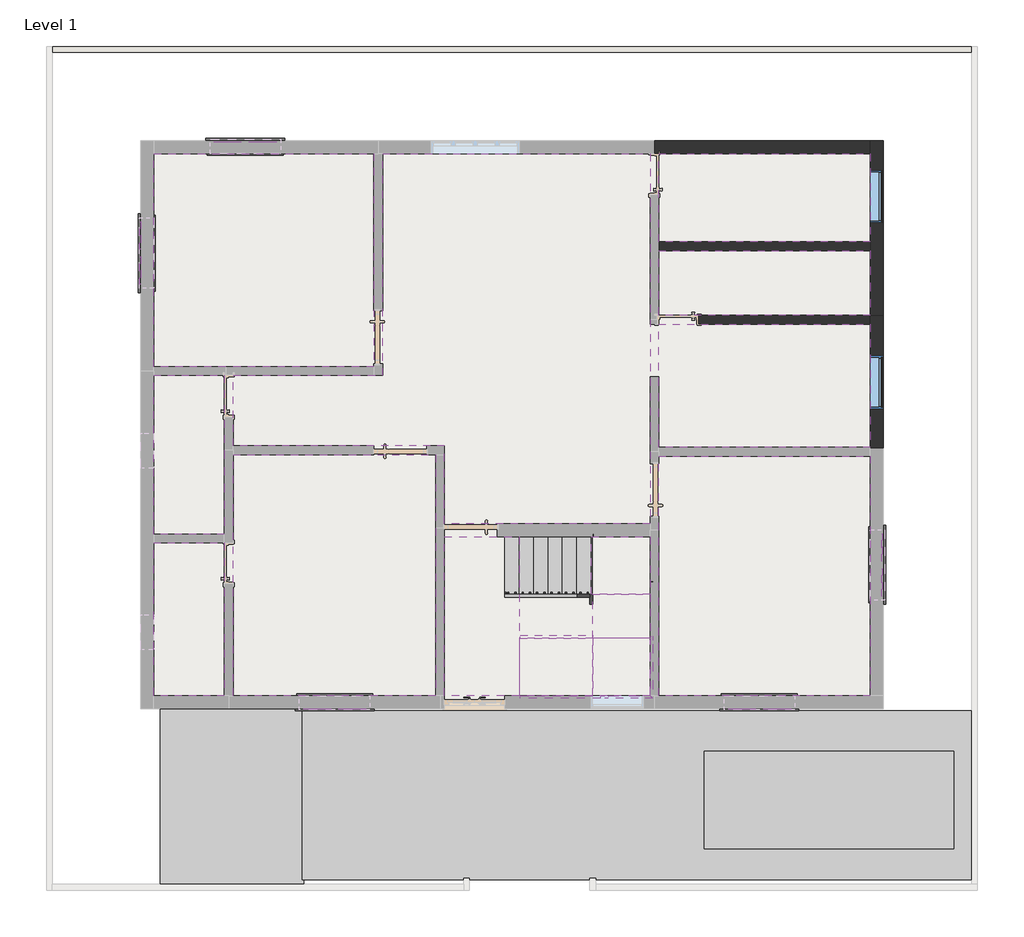
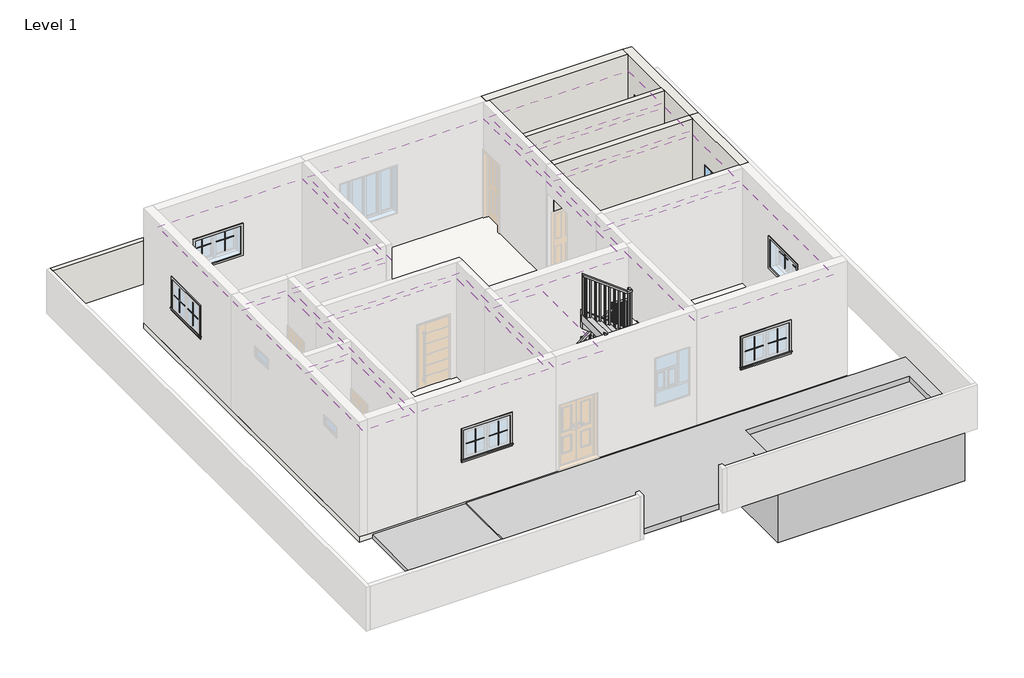
# One storey, part 2 of 2: 22 proxies, 10 coverings, 10 members, 6 walls, 3 slabs, 3 stair flights, 2 windows, 1 railing.
"""IFC4 building model written with IfcOpenShell, lengths in millimetres."""

from ifc_helpers import new_model, si_unit, frame, origin, origin_with_axes, place, context, project, spatial, polyline, outline, extrude, faceted_brep, transform, mapped, element, save
from components import generic_models_1_generic_models_1_4ef364dd, m_muntin_pattern_2x2_m_muntin_pattern_2x2_8d9e5da3, m_muntin_pattern_2x2_m_muntin_pattern_2x2_32a0f80e, m_trim_window_exterior_flat_with_sill_3a557199, m_trim_window_exterior_flat_with_sill_1a4b2e7c, m_trim_window_interior_flat_picture_frame_580345df, m_trim_window_interior_flat_picture_frame_7ff13b15, swimming_pool_swimming_pool_f5703ba1, non_monolithic_landing_f8b46ba6, non_monolithic_landing_0691aa35, stair_flight_50mm_tread_13mm_riser_519f3169, stair_flight_50mm_tread_13mm_riser_ecc54b48, stair_flight_50mm_tread_13mm_riser_ab1ff6a1, m_window_casement_double_sash_variable_3_661e274a

model = new_model("IFC4")

# Units and contexts
model_context = context("Model", 3, world=origin())
ifc_project = project(units=[si_unit("LENGTHUNIT", "METRE", prefix="MILLI")], contexts=[model_context])

# Site, building, storey
site = spatial("IfcSite", under=ifc_project)
building = spatial("IfcBuilding", under=site)
storey = spatial("IfcBuildingStorey", under=building, Name="Level 1", Elevation=0.0)

# Proxies
placement = place(None, origin())
generic_models_1_generic_models_1_shape = generic_models_1_generic_models_1_4ef364dd(model_context)
element("IfcBuildingElementProxy", 1, Name="Generic Models 1 : Generic Models 1", ObjectType="Generic Models 1 : Generic Models 1", at=placement, inside=storey, context=model_context, shape_type="MappedRepresentation", body=[
    mapped(generic_models_1_generic_models_1_shape, transform((0.0, 0.0, 0.0), x_axis=(1.0, 0.0, 0.0), y_axis=(0.0, 1.0, 0.0), z_axis=(0.0, 0.0, 1.0))),
])
m_muntin_pattern_2x2_m_muntin_pattern_2x2_shape = m_muntin_pattern_2x2_m_muntin_pattern_2x2_8d9e5da3(model_context)
element("IfcBuildingElementProxy", 2, Name="M_Muntin Pattern_2x2 : M_Muntin Pattern_2x2", ObjectType="M_Muntin Pattern_2x2 : M_Muntin Pattern_2x2", at=placement, inside=storey, context=model_context, shape_type="MappedRepresentation", body=[
    mapped(m_muntin_pattern_2x2_m_muntin_pattern_2x2_shape, transform((-16781.6669909, 5340.5131491, 1289.05), x_axis=(1.0, 0.0, 0.0), y_axis=(0.0, 1.0, 0.0), z_axis=(0.0, 0.0, 1.0))),
])
element("IfcBuildingElementProxy", 3, Name="M_Muntin Pattern_2x2 : M_Muntin Pattern_2x2", ObjectType="M_Muntin Pattern_2x2 : M_Muntin Pattern_2x2", at=placement, inside=storey, context=model_context, shape_type="MappedRepresentation", body=[
    mapped(m_muntin_pattern_2x2_m_muntin_pattern_2x2_shape, transform((-18281.8544909, 3098.9631491, 1289.05), x_axis=(0.0, 1.0, 0.0), y_axis=(-1.0, 0.0, 0.0), z_axis=(0.0, 0.0, 1.0))),
])
element("IfcBuildingElementProxy", 4, Name="M_Muntin Pattern_2x2 : M_Muntin Pattern_2x2", ObjectType="M_Muntin Pattern_2x2 : M_Muntin Pattern_2x2", at=placement, inside=storey, context=model_context, shape_type="MappedRepresentation", body=[
    mapped(m_muntin_pattern_2x2_m_muntin_pattern_2x2_shape, transform((-5448.5044909, -1687.3493509, 1289.05), x_axis=(0.0, -1.0, 0.0), y_axis=(1.0, 0.0, 0.0), z_axis=(0.0, 0.0, 1.0))),
])
element("IfcBuildingElementProxy", 5, Name="M_Muntin Pattern_2x2 : M_Muntin Pattern_2x2", ObjectType="M_Muntin Pattern_2x2 : M_Muntin Pattern_2x2", at=placement, inside=storey, context=model_context, shape_type="MappedRepresentation", body=[
    mapped(m_muntin_pattern_2x2_m_muntin_pattern_2x2_shape, transform((-7283.6544909, -4470.2368509, 1289.05), x_axis=(-1.0, 0.0, 0.0), y_axis=(0.0, -1.0, 0.0), z_axis=(0.0, 0.0, 1.0))),
])
element("IfcBuildingElementProxy", 6, Name="M_Muntin Pattern_2x2 : M_Muntin Pattern_2x2", ObjectType="M_Muntin Pattern_2x2 : M_Muntin Pattern_2x2", at=placement, inside=storey, context=model_context, shape_type="MappedRepresentation", body=[
    mapped(m_muntin_pattern_2x2_m_muntin_pattern_2x2_shape, transform((-14631.3982409, -4470.2368509, 1289.05), x_axis=(-1.0, 0.0, 0.0), y_axis=(0.0, -1.0, 0.0), z_axis=(0.0, 0.0, 1.0))),
])
m_muntin_pattern_2x2_m_muntin_pattern_2x2_2_shape = m_muntin_pattern_2x2_m_muntin_pattern_2x2_32a0f80e(model_context)
element("IfcBuildingElementProxy", 7, Name="M_Muntin Pattern_2x2 : M_Muntin Pattern_2x2", ObjectType="M_Muntin Pattern_2x2 : M_Muntin Pattern_2x2", at=placement, inside=storey, context=model_context, shape_type="MappedRepresentation", body=[
    mapped(m_muntin_pattern_2x2_m_muntin_pattern_2x2_2_shape, transform((-16175.2419909, 5340.5131491, 1289.05), x_axis=(-1.0, 0.0, 0.0), y_axis=(0.0, -1.0, 0.0), z_axis=(0.0, 0.0, 1.0))),
])
element("IfcBuildingElementProxy", 8, Name="M_Muntin Pattern_2x2 : M_Muntin Pattern_2x2", ObjectType="M_Muntin Pattern_2x2 : M_Muntin Pattern_2x2", at=placement, inside=storey, context=model_context, shape_type="MappedRepresentation", body=[
    mapped(m_muntin_pattern_2x2_m_muntin_pattern_2x2_2_shape, transform((-18281.8544909, 3705.3881491, 1289.05), x_axis=(0.0, -1.0, 0.0), y_axis=(1.0, 0.0, 0.0), z_axis=(0.0, 0.0, 1.0))),
])
element("IfcBuildingElementProxy", 9, Name="M_Muntin Pattern_2x2 : M_Muntin Pattern_2x2", ObjectType="M_Muntin Pattern_2x2 : M_Muntin Pattern_2x2", at=placement, inside=storey, context=model_context, shape_type="MappedRepresentation", body=[
    mapped(m_muntin_pattern_2x2_m_muntin_pattern_2x2_2_shape, transform((-5448.5044909, -2293.7743509, 1289.05), x_axis=(0.0, 1.0, 0.0), y_axis=(-1.0, 0.0, 0.0), z_axis=(0.0, 0.0, 1.0))),
])
element("IfcBuildingElementProxy", 10, Name="M_Muntin Pattern_2x2 : M_Muntin Pattern_2x2", ObjectType="M_Muntin Pattern_2x2 : M_Muntin Pattern_2x2", at=placement, inside=storey, context=model_context, shape_type="MappedRepresentation", body=[
    mapped(m_muntin_pattern_2x2_m_muntin_pattern_2x2_2_shape, transform((-7890.0794909, -4470.2368509, 1289.05), x_axis=(1.0, 0.0, 0.0), y_axis=(0.0, 1.0, 0.0), z_axis=(0.0, 0.0, 1.0))),
])
element("IfcBuildingElementProxy", 11, Name="M_Muntin Pattern_2x2 : M_Muntin Pattern_2x2", ObjectType="M_Muntin Pattern_2x2 : M_Muntin Pattern_2x2", at=placement, inside=storey, context=model_context, shape_type="MappedRepresentation", body=[
    mapped(m_muntin_pattern_2x2_m_muntin_pattern_2x2_2_shape, transform((-15237.8232409, -4470.2368509, 1289.05), x_axis=(1.0, 0.0, 0.0), y_axis=(0.0, 1.0, 0.0), z_axis=(0.0, 0.0, 1.0))),
])
m_trim_window_exterior_flat_with_sill_shape = m_trim_window_exterior_flat_with_sill_3a557199(model_context)
element("IfcBuildingElementProxy", 12, Name="M_Trim-Window-Exterior-Flat : with Sill", ObjectType="M_Trim-Window-Exterior-Flat : with Sill", at=placement, inside=storey, context=model_context, shape_type="MappedRepresentation", body=[
    mapped(m_trim_window_exterior_flat_with_sill_shape, transform((-18291.3794909, 3402.1756491, 2019.2), x_axis=(0.0, -1.0, 0.0), y_axis=(0.0, 0.0, 1.0), z_axis=(-1.0, 0.0, 0.0))),
])
element("IfcBuildingElementProxy", 13, Name="M_Trim-Window-Exterior-Flat : with Sill", ObjectType="M_Trim-Window-Exterior-Flat : with Sill", at=placement, inside=storey, context=model_context, shape_type="MappedRepresentation", body=[
    mapped(m_trim_window_exterior_flat_with_sill_shape, transform((-5438.9794909, -1990.5618509, 2019.2), x_axis=(0.0, 1.0, 0.0), y_axis=(0.0, 0.0, 1.0), z_axis=(1.0, 0.0, 0.0))),
])
element("IfcBuildingElementProxy", 14, Name="M_Trim-Window-Exterior-Flat : with Sill", ObjectType="M_Trim-Window-Exterior-Flat : with Sill", at=placement, inside=storey, context=model_context, shape_type="MappedRepresentation", body=[
    mapped(m_trim_window_exterior_flat_with_sill_shape, transform((-7586.8669909, -4479.7618509, 2019.2), x_axis=(1.0, 0.0, 0.0), y_axis=(0.0, 0.0, 1.0), z_axis=(0.0, -1.0, 0.0))),
])
element("IfcBuildingElementProxy", 15, Name="M_Trim-Window-Exterior-Flat : with Sill", ObjectType="M_Trim-Window-Exterior-Flat : with Sill", at=placement, inside=storey, context=model_context, shape_type="MappedRepresentation", body=[
    mapped(m_trim_window_exterior_flat_with_sill_shape, transform((-14934.6107409, -4479.7618509, 2019.2), x_axis=(1.0, 0.0, 0.0), y_axis=(0.0, 0.0, 1.0), z_axis=(0.0, -1.0, 0.0))),
])
m_trim_window_exterior_flat_with_sill_2_shape = m_trim_window_exterior_flat_with_sill_1a4b2e7c(model_context)
element("IfcBuildingElementProxy", 16, Name="M_Trim-Window-Exterior-Flat : with Sill", ObjectType="M_Trim-Window-Exterior-Flat : with Sill", at=placement, inside=storey, context=model_context, shape_type="MappedRepresentation", body=[
    mapped(m_trim_window_exterior_flat_with_sill_2_shape, transform((-16478.4544909, 5350.0381491, 2019.2), x_axis=(1.0, 0.0, 0.0), y_axis=(0.0, 0.0, -1.0), z_axis=(0.0, 1.0, 0.0))),
])
m_trim_window_interior_flat_picture_frame_shape = m_trim_window_interior_flat_picture_frame_580345df(model_context)
element("IfcBuildingElementProxy", 17, Name="M_Trim-Window-Interior-Flat : Picture Frame", ObjectType="M_Trim-Window-Interior-Flat : Picture Frame", at=placement, inside=storey, context=model_context, shape_type="MappedRepresentation", body=[
    mapped(m_trim_window_interior_flat_picture_frame_shape, transform((-18062.7794909, 3402.1756491, 2019.2), x_axis=(0.0, 1.0, 0.0), y_axis=(0.0, 0.0, 1.0), z_axis=(1.0, 0.0, 0.0))),
])
element("IfcBuildingElementProxy", 18, Name="M_Trim-Window-Interior-Flat : Picture Frame", ObjectType="M_Trim-Window-Interior-Flat : Picture Frame", at=placement, inside=storey, context=model_context, shape_type="MappedRepresentation", body=[
    mapped(m_trim_window_interior_flat_picture_frame_shape, transform((-5667.5794909, -1990.5618509, 2019.2), x_axis=(0.0, -1.0, 0.0), y_axis=(0.0, 0.0, 1.0), z_axis=(-1.0, 0.0, 0.0))),
])
element("IfcBuildingElementProxy", 19, Name="M_Trim-Window-Interior-Flat : Picture Frame", ObjectType="M_Trim-Window-Interior-Flat : Picture Frame", at=placement, inside=storey, context=model_context, shape_type="MappedRepresentation", body=[
    mapped(m_trim_window_interior_flat_picture_frame_shape, transform((-7586.8669909, -4251.1618509, 2019.2), x_axis=(-1.0, 0.0, 0.0), y_axis=(0.0, 0.0, 1.0), z_axis=(0.0, 1.0, 0.0))),
])
element("IfcBuildingElementProxy", 20, Name="M_Trim-Window-Interior-Flat : Picture Frame", ObjectType="M_Trim-Window-Interior-Flat : Picture Frame", at=placement, inside=storey, context=model_context, shape_type="MappedRepresentation", body=[
    mapped(m_trim_window_interior_flat_picture_frame_shape, transform((-14934.6107409, -4251.1618509, 2019.2), x_axis=(-1.0, 0.0, 0.0), y_axis=(0.0, 0.0, 1.0), z_axis=(0.0, 1.0, 0.0))),
])
m_trim_window_interior_flat_picture_frame_2_shape = m_trim_window_interior_flat_picture_frame_7ff13b15(model_context)
element("IfcBuildingElementProxy", 21, Name="M_Trim-Window-Interior-Flat : Picture Frame", ObjectType="M_Trim-Window-Interior-Flat : Picture Frame", at=placement, inside=storey, context=model_context, shape_type="MappedRepresentation", body=[
    mapped(m_trim_window_interior_flat_picture_frame_2_shape, transform((-16478.4544909, 5121.4381491, 2019.2), x_axis=(-1.0, 0.0, 0.0), y_axis=(0.0, 0.0, -1.0), z_axis=(0.0, -1.0, 0.0))),
])
swimming_pool_swimming_pool_shape = swimming_pool_swimming_pool_f5703ba1(model_context)
element("IfcBuildingElementProxy", 22, Name="SWIMMING POOL : SWIMMING POOL", ObjectType="SWIMMING POOL : SWIMMING POOL", at=placement, inside=storey, context=model_context, shape_type="MappedRepresentation", body=[
    mapped(swimming_pool_swimming_pool_shape, transform((0.0, 76.2, 0.0), x_axis=(1.0, 0.0, 0.0), y_axis=(0.0, 1.0, 0.0), z_axis=(0.0, 0.0, 1.0))),
])

# Coverings
element("IfcCovering", 23, ObjectType="Plain", at=placement, inside=storey, context=model_context, shape_type="SweptSolid", body=[
    extrude(outline(polyline([(-18062.7794909, 1438.4381491), (-18062.7794909, 5121.4381491), (-14252.7794909, 5121.4381491), (-14252.7794909, 1438.4381491), (-16818.1794909, 1438.4381491), (-18062.7794909, 1438.4381491)])), frame((0.0, 0.0, 2743.2), z_axis=(0.0, 0.0, 1.0), x_axis=(1.0, 0.0, 0.0)), (0.0, 0.0, 1.0), 57.0),
])
element("IfcCovering", 24, ObjectType="Plain", at=placement, inside=storey, context=model_context, shape_type="SweptSolid", body=[
    extrude(outline(polyline([(-16691.1794909, 1286.0381491), (-14100.3794909, 1286.0381491), (-14100.3794909, 5121.4381491), (-9477.5794909, 5121.4381491), (-9477.5794909, 2251.2381491), (-9477.5794909, -34.7618509), (-9477.5794909, -1279.3618509), (-13033.5794909, -1279.3618509), (-13033.5794909, 66.8381491), (-16691.1794909, 66.8381491), (-16691.1794909, 1286.0381491)])), frame((0.0, 0.0, 2743.2), z_axis=(0.0, 0.0, 1.0), x_axis=(1.0, 0.0, 0.0)), (0.0, 0.0, 1.0), 57.0),
])
element("IfcCovering", 25, ObjectType="Plain", at=placement, inside=storey, context=model_context, shape_type="SweptSolid", body=[
    extrude(outline(polyline([(-9325.1794909, -110.9618509), (-5667.5794909, -110.9618509), (-5667.5794909, -4251.1618509), (-9325.1794909, -4251.1618509), (-9325.1794909, -1393.6618509), (-9325.1794909, -110.9618509)])), frame((0.0, 0.0, 2743.2), z_axis=(0.0, 0.0, 1.0), x_axis=(1.0, 0.0, 0.0)), (0.0, 0.0, 1.0), 57.0),
])
element("IfcCovering", 26, ObjectType="Plain", at=placement, inside=storey, context=model_context, shape_type="SweptSolid", body=[
    extrude(outline(polyline([(-9325.1794909, 2175.0381491), (-5667.5794909, 2175.0381491), (-5667.5794909, 41.4381491), (-9325.1794909, 41.4381491), (-9325.1794909, 2175.0381491)])), frame((0.0, 0.0, 2743.2), z_axis=(0.0, 0.0, 1.0), x_axis=(1.0, 0.0, 0.0)), (0.0, 0.0, 1.0), 57.0),
])
element("IfcCovering", 27, ObjectType="Plain", at=placement, inside=storey, context=model_context, shape_type="SweptSolid", body=[
    extrude(outline(polyline([(-9325.1794909, 3445.0381491), (-5667.5794909, 3445.0381491), (-5667.5794909, 2327.4381491), (-9325.1794909, 2327.4381491), (-9325.1794909, 3445.0381491)])), frame((0.0, 0.0, 2743.2), z_axis=(0.0, 0.0, 1.0), x_axis=(1.0, 0.0, 0.0)), (0.0, 0.0, 1.0), 57.0),
])
element("IfcCovering", 28, ObjectType="Plain", at=placement, inside=storey, context=model_context, shape_type="SweptSolid", body=[
    extrude(outline(polyline([(-9325.1794909, 5121.4381491), (-5667.5794909, 5121.4381491), (-5667.5794909, 3597.4381491), (-9325.1794909, 3597.4381491), (-9325.1794909, 5121.4381491)])), frame((0.0, 0.0, 2743.2), z_axis=(0.0, 0.0, 1.0), x_axis=(1.0, 0.0, 0.0)), (0.0, 0.0, 1.0), 57.0),
])
element("IfcCovering", 29, ObjectType="Plain", at=placement, inside=storey, context=model_context, shape_type="SweptSolid", body=[
    extrude(outline(polyline([(-13185.9794909, -4251.1618509), (-16691.1794909, -4251.1618509), (-16691.1794909, -85.5618509), (-13185.9794909, -85.5618509), (-13185.9794909, -1355.5618509), (-13185.9794909, -4251.1618509)])), frame((0.0, 0.0, 2743.2), z_axis=(0.0, 0.0, 1.0), x_axis=(1.0, 0.0, 0.0)), (0.0, 0.0, 1.0), 57.0),
])
element("IfcCovering", 30, ObjectType="Plain", at=placement, inside=storey, context=model_context, shape_type="SweptSolid", body=[
    extrude(outline(polyline([(-16843.5794909, 1286.0381491), (-16843.5794909, -9.3618509), (-16843.5794909, -1457.1618509), (-18062.7794909, -1457.1618509), (-18062.7794909, 1286.0381491), (-16843.5794909, 1286.0381491)])), frame((0.0, 0.0, 2743.2), z_axis=(0.0, 0.0, 1.0), x_axis=(1.0, 0.0, 0.0)), (0.0, 0.0, 1.0), 57.0),
])
element("IfcCovering", 31, ObjectType="Plain", at=placement, inside=storey, context=model_context, shape_type="SweptSolid", body=[
    extrude(outline(polyline([(-16843.5794909, -1609.5618509), (-16843.5794909, -4251.1618509), (-18062.7794909, -4251.1618509), (-18062.7794909, -1609.5618509), (-16843.5794909, -1609.5618509)])), frame((0.0, 0.0, 2743.2), z_axis=(0.0, 0.0, 1.0), x_axis=(1.0, 0.0, 0.0)), (0.0, 0.0, 1.0), 57.0),
])
element("IfcCovering", 32, ObjectType="Plain", at=placement, inside=storey, context=model_context, shape_type="SweptSolid", body=[
    extrude(outline(polyline([(-13033.5794909, -4251.1618509), (-13033.5794909, -1507.9618509), (-11738.1794909, -1507.9618509), (-11738.1794909, -4251.1618509), (-13033.5794909, -4251.1618509)])), frame((0.0, 0.0, 2743.2), z_axis=(0.0, 0.0, 1.0), x_axis=(1.0, 0.0, 0.0)), (0.0, 0.0, 1.0), 57.0),
])

# Members
element("IfcMember", 33, ObjectType="Stringer - 50mm Width", at=placement, inside=storey, context=model_context, shape_type="SweptSolid", body=[
    extrude(outline(polyline([(253.5429417, -11992.1794909), (0.0, -11992.1794909), (0.0, -11663.9259909), (967.8117647, -10378.7116427), (1367.8117647, -10512.4761733), (253.5429417, -11992.1794909)])), frame((0.0, -1507.9618509, 0.0), z_axis=(0.0, 1.0, 0.0), x_axis=(0.0, 0.0, 1.0)), (0.0, 0.0, 1.0), 50.0),
])
element("IfcMember", 34, ObjectType="Stringer - 50mm Width", at=placement, inside=storey, context=model_context, shape_type="SweptSolid", body=[
    extrude(outline(polyline([(253.5429417, -11992.1794909), (0.0, -11992.1794909), (0.0, -11663.9259909), (862.7875526, -10518.1794909), (1363.5169652, -10518.1794909), (253.5429417, -11992.1794909)])), frame((0.0, -2548.5618509, 0.0), z_axis=(0.0, 1.0, 0.0), x_axis=(0.0, 0.0, 1.0)), (0.0, 0.0, 1.0), 50.0),
])
element("IfcMember", 35, ObjectType="Stringer - 50mm Width", at=placement, inside=storey, context=model_context, shape_type="SweptSolid", body=[
    extrude(outline(polyline([(-2228.2651685, 1367.8117647), (-2362.029699, 967.8117647), (-3362.029699, 1720.8470588), (-3228.2651685, 2120.8470588), (-2228.2651685, 1367.8117647)])), frame((-9477.5794909, 0.0, 0.0), z_axis=(1.0, 0.0, 0.0), x_axis=(0.0, 1.0, 0.0)), (0.0, 0.0, 1.0), 50.0),
])
element("IfcMember", 36, ObjectType="Stringer - 50mm Width", at=placement, inside=storey, context=model_context, shape_type="SweptSolid", body=[
    extrude(outline(polyline([(-2498.5618509, 1571.3547064), (-2498.5618509, 1070.6252938), (-3210.5618509, 1606.7864232), (-3210.5618509, 2107.5158358), (-2498.5618509, 1571.3547064)])), frame((-10518.1794909, 0.0, 0.0), z_axis=(1.0, 0.0, 0.0), x_axis=(0.0, 1.0, 0.0)), (0.0, 0.0, 1.0), 50.0),
])
element("IfcMember", 37, ObjectType="Stringer - 50mm Width", at=placement, inside=storey, context=model_context, shape_type="Brep", body=[
    faceted_brep([(-9477.5794909, -2228.2651685, 1367.8117647), (-9427.5794909, -2228.2651685, 1367.8117647), (-9427.5794909, -1457.9618509, 1367.8117647), (-9477.5794909, -1507.9618509, 1367.8117647), (-9477.5794909, -2362.029699, 967.8117647), (-9477.5794909, -1507.9618509, 967.8117647), (-9427.5794909, -2362.029699, 967.8117647), (-9427.5794909, -1457.9618509, 967.8117647)], [[[0, 1, 2, 3]], [[4, 0, 3, 5]], [[6, 4, 5, 7]], [[1, 6, 7, 2]], [[1, 0, 4, 6]], [[2, 7, 5, 3]]]),
])
element("IfcMember", 38, ObjectType="Stringer - 50mm Width", at=placement, inside=storey, context=model_context, shape_type="Brep", body=[
    faceted_brep([(-9477.5794909, -1507.9618509, 1367.8117647), (-9427.5794909, -1457.9618509, 1367.8117647), (-10512.4761733, -1457.9618509, 1367.8117647), (-10512.4761733, -1507.9618509, 1367.8117647), (-9477.5794909, -1507.9618509, 967.8117647), (-10378.7116427, -1507.9618509, 967.8117647), (-9427.5794909, -1457.9618509, 967.8117647), (-10378.7116427, -1457.9618509, 967.8117647)], [[[0, 1, 2, 3]], [[4, 0, 3, 5]], [[6, 4, 5, 7]], [[1, 6, 7, 2]], [[1, 0, 4, 6]], [[2, 7, 5, 3]]]),
])
element("IfcMember", 39, ObjectType="Stringer - 50mm Width", at=placement, inside=storey, context=model_context, shape_type="SweptSolid", body=[
    extrude(outline(polyline([(1720.8470588, -10331.6473391), (2120.8470588, -10197.8828085), (3265.6841182, -11718.1794909), (2764.9547056, -11718.1794909), (1720.8470588, -10331.6473391)])), frame((0.0, -4301.1618509, 0.0), z_axis=(0.0, 1.0, 0.0), x_axis=(0.0, 0.0, 1.0)), (0.0, 0.0, 1.0), 50.0),
])
element("IfcMember", 40, ObjectType="Stringer - 50mm Width", at=placement, inside=storey, context=model_context, shape_type="SweptSolid", body=[
    extrude(outline(polyline([(1823.6605879, -10468.1794909), (2324.3900005, -10468.1794909), (3265.6841182, -11718.1794909), (2764.9547056, -11718.1794909), (1823.6605879, -10468.1794909)])), frame((0.0, -3260.5618509, 0.0), z_axis=(0.0, 1.0, 0.0), x_axis=(0.0, 0.0, 1.0)), (0.0, 0.0, 1.0), 50.0),
])
element("IfcMember", 41, ObjectType="Stringer - 50mm Width", at=placement, inside=storey, context=model_context, shape_type="Brep", body=[
    faceted_brep([(-10197.8828085, -4251.1618509, 2120.8470588), (-10197.8828085, -4301.1618509, 2120.8470588), (-9427.5794909, -4301.1618509, 2120.8470588), (-9477.5794909, -4251.1618509, 2120.8470588), (-10331.6473391, -4251.1618509, 1720.8470588), (-9477.5794909, -4251.1618509, 1720.8470588), (-10331.6473391, -4301.1618509, 1720.8470588), (-9427.5794909, -4301.1618509, 1720.8470588)], [[[0, 1, 2, 3]], [[4, 0, 3, 5]], [[6, 4, 5, 7]], [[1, 6, 7, 2]], [[1, 0, 4, 6]], [[2, 7, 5, 3]]]),
])
element("IfcMember", 42, ObjectType="Stringer - 50mm Width", at=placement, inside=storey, context=model_context, shape_type="Brep", body=[
    faceted_brep([(-9477.5794909, -4251.1618509, 2120.8470588), (-9427.5794909, -4301.1618509, 2120.8470588), (-9427.5794909, -3228.2651685, 2120.8470588), (-9477.5794909, -3228.2651685, 2120.8470588), (-9477.5794909, -4251.1618509, 1720.8470588), (-9477.5794909, -3362.029699, 1720.8470588), (-9427.5794909, -4301.1618509, 1720.8470588), (-9427.5794909, -3362.029699, 1720.8470588)], [[[0, 1, 2, 3]], [[4, 0, 3, 5]], [[6, 4, 5, 7]], [[1, 6, 7, 2]], [[1, 0, 4, 6]], [[2, 7, 5, 3]]]),
])

# Railing
element("IfcRailing", 43, ObjectType="1100mm", at=placement, inside=storey, context=model_context, shape_type="SolidModel", body=[
    faceted_brep([(-11992.1794909, -2448.1618509, 1288.2588235), (-11992.1794909, -2448.1618509, 1225.667647), (-11992.1794909, -2498.1618509, 1225.667647), (-11992.1794909, -2498.1618509, 1288.2588235), (-10492.1794909, -2448.1618509, 2417.8117647), (-10475.4589246, -2448.1618509, 2367.8117647), (-10475.4589246, -2498.1618509, 2367.8117647), (-10492.1794909, -2498.1618509, 2417.8117647), (-10467.7794909, -2448.1618509, 2417.8117647), (-10467.7794909, -2498.1618509, 2417.8117647), (-10417.7794909, -2498.1618509, 2367.8117647), (-10417.7794909, -2448.1618509, 2367.8117647)], [[[0, 1, 2, 3]], [[1, 0, 4, 5]], [[2, 1, 5, 6]], [[3, 2, 6, 7]], [[0, 3, 7, 4]], [[8, 9, 10, 11]], [[5, 4, 8, 11]], [[6, 5, 11, 10]], [[7, 6, 10, 9]], [[4, 7, 9, 8]]]),
    faceted_brep([(-10467.7794909, -2448.1618509, 2417.8117647), (-10417.7794909, -2448.1618509, 2367.8117647), (-10417.7794909, -2498.1618509, 2367.8117647), (-10467.7794909, -2498.1618509, 2417.8117647), (-10467.7794909, -2448.1618509, 2568.1176094), (-10467.7794909, -2498.1618509, 2543.1781975), (-10417.7794909, -2498.1618509, 2543.1781975), (-10417.7794909, -2448.1618509, 2568.1176094)], [[[0, 1, 2, 3]], [[4, 5, 6, 7]], [[1, 0, 4, 7]], [[2, 1, 7, 6]], [[3, 2, 6, 5]], [[0, 3, 5, 4]]]),
    faceted_brep([(-10417.7794909, -2448.1618509, 2568.1176094), (-10417.7794909, -2498.1618509, 2543.1781975), (-10467.7794909, -2498.1618509, 2543.1781975), (-10467.7794909, -2448.1618509, 2568.1176094), (-10417.7794909, -3185.9618509, 3123.7070494), (-10417.7794909, -3235.9618509, 3098.7676375), (-10467.7794909, -3235.9618509, 3098.7676375), (-10467.7794909, -3185.9618509, 3123.7070494), (-10417.7794909, -3185.9618509, 3415.2823153), (-10417.7794909, -3235.9618509, 3365.2823153), (-10467.7794909, -3235.9618509, 3365.2823153), (-10467.7794909, -3185.9618509, 3415.2823153), (-10417.7794909, -3310.9618509, 3415.2823153), (-10417.7794909, -3310.9618509, 3365.2823153), (-10467.7794909, -3260.9618509, 3365.2823153), (-10467.7794909, -3260.9618509, 3415.2823153), (-10542.7794909, -3310.9618509, 3415.2823153), (-10559.5000572, -3310.9618509, 3365.2823153), (-10559.5000572, -3260.9618509, 3365.2823153), (-10542.7794909, -3260.9618509, 3415.2823153), (-11718.1794909, -3310.9618509, 4300.4), (-11718.1794909, -3260.9618509, 4300.4), (-11718.1794909, -3260.9618509, 4237.8088234), (-11718.1794909, -3310.9618509, 4237.8088234)], [[[0, 1, 2, 3]], [[1, 0, 4, 5]], [[2, 1, 5, 6]], [[3, 2, 6, 7]], [[0, 3, 7, 4]], [[5, 4, 8, 9]], [[6, 5, 9, 10]], [[7, 6, 10, 11]], [[4, 7, 11, 8]], [[9, 8, 12, 13]], [[10, 9, 13, 14]], [[11, 10, 14, 15]], [[8, 11, 15, 12]], [[13, 12, 16, 17]], [[14, 13, 17, 18]], [[15, 14, 18, 19]], [[12, 15, 19, 16]], [[20, 21, 22, 23]], [[17, 16, 20, 23]], [[18, 17, 23, 22]], [[19, 18, 22, 21]], [[16, 19, 21, 20]]]),
    extrude(outline(polyline([(3012.1411765, -11617.7794909), (4162.2040799, -11617.7794909), (4181.0299622, -11642.7794909), (3012.1411765, -11642.7794909), (3012.1411765, -11617.7794909)])), frame((0.0, -3298.4618509, 0.0), z_axis=(0.0, 1.0, 0.0), x_axis=(0.0, 0.0, 1.0)), (0.0, 0.0, 1.0), 25.0),
    extrude(outline(polyline([(3012.1411765, -11492.7794909), (4068.0746681, -11492.7794909), (4086.9005505, -11517.7794909), (3012.1411765, -11517.7794909), (3012.1411765, -11492.7794909)])), frame((0.0, -3298.4618509, 0.0), z_axis=(0.0, 1.0, 0.0), x_axis=(0.0, 0.0, 1.0)), (0.0, 0.0, 1.0), 25.0),
    extrude(outline(polyline([(2823.8823529, -11367.7794909), (3973.9452564, -11367.7794909), (3992.7711387, -11392.7794909), (2823.8823529, -11392.7794909), (2823.8823529, -11367.7794909)])), frame((0.0, -3298.4618509, 0.0), z_axis=(0.0, 1.0, 0.0), x_axis=(0.0, 0.0, 1.0)), (0.0, 0.0, 1.0), 25.0),
    extrude(outline(polyline([(2823.8823529, -11242.7794909), (3879.8158446, -11242.7794909), (3898.641727, -11267.7794909), (2823.8823529, -11267.7794909), (2823.8823529, -11242.7794909)])), frame((0.0, -3298.4618509, 0.0), z_axis=(0.0, 1.0, 0.0), x_axis=(0.0, 0.0, 1.0)), (0.0, 0.0, 1.0), 25.0),
    extrude(outline(polyline([(2635.6235294, -11117.7794909), (3785.6864328, -11117.7794909), (3804.5123152, -11142.7794909), (2635.6235294, -11142.7794909), (2635.6235294, -11117.7794909)])), frame((0.0, -3298.4618509, 0.0), z_axis=(0.0, 1.0, 0.0), x_axis=(0.0, 0.0, 1.0)), (0.0, 0.0, 1.0), 25.0),
    extrude(outline(polyline([(2635.6235294, -10992.7794909), (3691.5570211, -10992.7794909), (3710.3829034, -11017.7794909), (2635.6235294, -11017.7794909), (2635.6235294, -10992.7794909)])), frame((0.0, -3298.4618509, 0.0), z_axis=(0.0, 1.0, 0.0), x_axis=(0.0, 0.0, 1.0)), (0.0, 0.0, 1.0), 25.0),
    extrude(outline(polyline([(2447.3647059, -10867.7794909), (3597.4276093, -10867.7794909), (3616.2534917, -10892.7794909), (2447.3647059, -10892.7794909), (2447.3647059, -10867.7794909)])), frame((0.0, -3298.4618509, 0.0), z_axis=(0.0, 1.0, 0.0), x_axis=(0.0, 0.0, 1.0)), (0.0, 0.0, 1.0), 25.0),
    extrude(outline(polyline([(2447.3647059, -10742.7794909), (3503.2981975, -10742.7794909), (3522.1240799, -10767.7794909), (2447.3647059, -10767.7794909), (2447.3647059, -10742.7794909)])), frame((0.0, -3298.4618509, 0.0), z_axis=(0.0, 1.0, 0.0), x_axis=(0.0, 0.0, 1.0)), (0.0, 0.0, 1.0), 25.0),
    extrude(outline(polyline([(2259.1058824, -10617.7794909), (3409.1687858, -10617.7794909), (3427.9946681, -10642.7794909), (2259.1058824, -10642.7794909), (2259.1058824, -10617.7794909)])), frame((0.0, -3298.4618509, 0.0), z_axis=(0.0, 1.0, 0.0), x_axis=(0.0, 0.0, 1.0)), (0.0, 0.0, 1.0), 25.0),
    extrude(outline(polyline([(-10492.7794909, -3273.4618509), (-10492.7794909, -3298.4618509), (-10517.7794909, -3298.4618509), (-10517.7794909, -3273.4618509), (-10492.7794909, -3273.4618509)])), frame((0.0, 0.0, 2259.1058824), z_axis=(0.0, 0.0, 1.0), x_axis=(1.0, 0.0, 0.0)), (0.0, 0.0, 1.0), 1106.1764329),
    extrude(outline(polyline([(-3148.1618509, 3032.6511387), (-3148.1618509, 1882.5882353), (-3173.1618509, 1882.5882353), (-3173.1618509, 3051.4770211), (-3148.1618509, 3032.6511387)])), frame((-10455.2794909, 0.0, 0.0), z_axis=(1.0, 0.0, 0.0), x_axis=(0.0, 1.0, 0.0)), (0.0, 0.0, 1.0), 25.0),
    extrude(outline(polyline([(-3023.1618509, 2938.521727), (-3023.1618509, 1882.5882353), (-3048.1618509, 1882.5882353), (-3048.1618509, 2957.3476093), (-3023.1618509, 2938.521727)])), frame((-10455.2794909, 0.0, 0.0), z_axis=(1.0, 0.0, 0.0), x_axis=(0.0, 1.0, 0.0)), (0.0, 0.0, 1.0), 25.0),
    extrude(outline(polyline([(-2898.1618509, 2844.3923152), (-2898.1618509, 1694.3294118), (-2923.1618509, 1694.3294118), (-2923.1618509, 2863.2181975), (-2898.1618509, 2844.3923152)])), frame((-10455.2794909, 0.0, 0.0), z_axis=(1.0, 0.0, 0.0), x_axis=(0.0, 1.0, 0.0)), (0.0, 0.0, 1.0), 25.0),
    extrude(outline(polyline([(-2773.1618509, 2750.2629034), (-2773.1618509, 1694.3294118), (-2798.1618509, 1694.3294118), (-2798.1618509, 2769.0887858), (-2773.1618509, 2750.2629034)])), frame((-10455.2794909, 0.0, 0.0), z_axis=(1.0, 0.0, 0.0), x_axis=(0.0, 1.0, 0.0)), (0.0, 0.0, 1.0), 25.0),
    extrude(outline(polyline([(-2648.1618509, 2656.1334917), (-2648.1618509, 1506.0705882), (-2673.1618509, 1506.0705882), (-2673.1618509, 2674.959374), (-2648.1618509, 2656.1334917)])), frame((-10455.2794909, 0.0, 0.0), z_axis=(1.0, 0.0, 0.0), x_axis=(0.0, 1.0, 0.0)), (0.0, 0.0, 1.0), 25.0),
    extrude(outline(polyline([(-2523.1618509, 2562.0040799), (-2523.1618509, 1506.0705882), (-2548.1618509, 1506.0705882), (-2548.1618509, 2580.8299622), (-2523.1618509, 2562.0040799)])), frame((-10455.2794909, 0.0, 0.0), z_axis=(1.0, 0.0, 0.0), x_axis=(0.0, 1.0, 0.0)), (0.0, 0.0, 1.0), 25.0),
    extrude(outline(polyline([(2298.7429411, -10567.1794909), (1129.5529412, -10567.1794909), (1129.5529412, -10542.1794909), (2317.5688234, -10542.1794909), (2298.7429411, -10567.1794909)])), frame((0.0, -2485.6618509, 0.0), z_axis=(0.0, 1.0, 0.0), x_axis=(0.0, 0.0, 1.0)), (0.0, 0.0, 1.0), 25.0),
    extrude(outline(polyline([(2204.6135293, -10692.1794909), (1129.5529412, -10692.1794909), (1129.5529412, -10667.1794909), (2223.4394117, -10667.1794909), (2204.6135293, -10692.1794909)])), frame((0.0, -2485.6618509, 0.0), z_axis=(0.0, 1.0, 0.0), x_axis=(0.0, 0.0, 1.0)), (0.0, 0.0, 1.0), 25.0),
    extrude(outline(polyline([(2110.4841175, -10817.1794909), (941.2941176, -10817.1794909), (941.2941176, -10792.1794909), (2129.3099999, -10792.1794909), (2110.4841175, -10817.1794909)])), frame((0.0, -2485.6618509, 0.0), z_axis=(0.0, 1.0, 0.0), x_axis=(0.0, 0.0, 1.0)), (0.0, 0.0, 1.0), 25.0),
    extrude(outline(polyline([(2016.3547058, -10942.1794909), (941.2941176, -10942.1794909), (941.2941176, -10917.1794909), (2035.1805881, -10917.1794909), (2016.3547058, -10942.1794909)])), frame((0.0, -2485.6618509, 0.0), z_axis=(0.0, 1.0, 0.0), x_axis=(0.0, 0.0, 1.0)), (0.0, 0.0, 1.0), 25.0),
    extrude(outline(polyline([(1922.225294, -11067.1794909), (753.0352941, -11067.1794909), (753.0352941, -11042.1794909), (1941.0511764, -11042.1794909), (1922.225294, -11067.1794909)])), frame((0.0, -2485.6618509, 0.0), z_axis=(0.0, 1.0, 0.0), x_axis=(0.0, 0.0, 1.0)), (0.0, 0.0, 1.0), 25.0),
    extrude(outline(polyline([(1828.0958822, -11192.1794909), (753.0352941, -11192.1794909), (753.0352941, -11167.1794909), (1846.9217646, -11167.1794909), (1828.0958822, -11192.1794909)])), frame((0.0, -2485.6618509, 0.0), z_axis=(0.0, 1.0, 0.0), x_axis=(0.0, 0.0, 1.0)), (0.0, 0.0, 1.0), 25.0),
    extrude(outline(polyline([(1733.9664705, -11317.1794909), (564.7764706, -11317.1794909), (564.7764706, -11292.1794909), (1752.7923528, -11292.1794909), (1733.9664705, -11317.1794909)])), frame((0.0, -2485.6618509, 0.0), z_axis=(0.0, 1.0, 0.0), x_axis=(0.0, 0.0, 1.0)), (0.0, 0.0, 1.0), 25.0),
    extrude(outline(polyline([(1639.8370587, -11442.1794909), (564.7764706, -11442.1794909), (564.7764706, -11417.1794909), (1658.6629411, -11417.1794909), (1639.8370587, -11442.1794909)])), frame((0.0, -2485.6618509, 0.0), z_axis=(0.0, 1.0, 0.0), x_axis=(0.0, 0.0, 1.0)), (0.0, 0.0, 1.0), 25.0),
    extrude(outline(polyline([(1545.707647, -11567.1794909), (376.5176471, -11567.1794909), (376.5176471, -11542.1794909), (1564.5335293, -11542.1794909), (1545.707647, -11567.1794909)])), frame((0.0, -2485.6618509, 0.0), z_axis=(0.0, 1.0, 0.0), x_axis=(0.0, 0.0, 1.0)), (0.0, 0.0, 1.0), 25.0),
    extrude(outline(polyline([(1451.5782352, -11692.1794909), (376.5176471, -11692.1794909), (376.5176471, -11667.1794909), (1470.4041175, -11667.1794909), (1451.5782352, -11692.1794909)])), frame((0.0, -2485.6618509, 0.0), z_axis=(0.0, 1.0, 0.0), x_axis=(0.0, 0.0, 1.0)), (0.0, 0.0, 1.0), 25.0),
    extrude(outline(polyline([(1357.4488234, -11817.1794909), (188.2588235, -11817.1794909), (188.2588235, -11792.1794909), (1376.2747058, -11792.1794909), (1357.4488234, -11817.1794909)])), frame((0.0, -2485.6618509, 0.0), z_axis=(0.0, 1.0, 0.0), x_axis=(0.0, 0.0, 1.0)), (0.0, 0.0, 1.0), 25.0),
    extrude(outline(polyline([(1263.3194117, -11942.1794909), (188.2588235, -11942.1794909), (188.2588235, -11917.1794909), (1282.145294, -11917.1794909), (1263.3194117, -11942.1794909)])), frame((0.0, -2485.6618509, 0.0), z_axis=(0.0, 1.0, 0.0), x_axis=(0.0, 0.0, 1.0)), (0.0, 0.0, 1.0), 25.0),
    extrude(outline(polyline([(-10455.2794909, -3273.4618509), (-10430.2794909, -3273.4618509), (-10430.2794909, -3298.4618509), (-10455.2794909, -3298.4618509), (-10455.2794909, -3273.4618509)])), frame((0.0, 0.0, 2070.8470588), z_axis=(0.0, 0.0, 1.0), x_axis=(1.0, 0.0, 0.0)), (0.0, 0.0, 1.0), 1294.4352565),
    extrude(outline(polyline([(-10455.2794909, -3236.0618509), (-10430.2794909, -3236.0618509), (-10430.2794909, -3261.0618509), (-10455.2794909, -3261.0618509), (-10455.2794909, -3236.0618509)])), frame((0.0, 0.0, 2070.8470588), z_axis=(0.0, 0.0, 1.0), x_axis=(1.0, 0.0, 0.0)), (0.0, 0.0, 1.0), 1294.4352565),
    extrude(outline(polyline([(-10455.2794909, -2485.6618509), (-10455.2794909, -2460.6618509), (-10430.2794909, -2460.6618509), (-10430.2794909, -2485.6618509), (-10455.2794909, -2485.6618509)])), frame((0.0, 0.0, 1317.8117647), z_axis=(0.0, 0.0, 1.0), x_axis=(1.0, 0.0, 0.0)), (0.0, 0.0, 1.0), 1050.0),
    extrude(outline(polyline([(2345.807647, -10504.6794909), (1317.8117647, -10504.6794909), (1317.8117647, -10479.6794909), (2364.6335293, -10479.6794909), (2345.807647, -10504.6794909)])), frame((0.0, -2485.6618509, 0.0), z_axis=(0.0, 1.0, 0.0), x_axis=(0.0, 0.0, 1.0)), (0.0, 0.0, 1.0), 25.0),
    extrude(outline(polyline([(3012.1411765, -11693.1794909), (4218.9829411, -11693.1794909), (4237.8088234, -11718.1794909), (3012.1411765, -11718.1794909), (3012.1411765, -11693.1794909)])), frame((0.0, -3298.4618509, 0.0), z_axis=(0.0, 1.0, 0.0), x_axis=(0.0, 0.0, 1.0)), (0.0, 0.0, 1.0), 25.0),
    extrude(outline(polyline([(1225.667647, -11992.1794909), (188.2588235, -11992.1794909), (188.2588235, -11967.1794909), (1244.4935293, -11967.1794909), (1225.667647, -11992.1794909)])), frame((0.0, -2485.6618509, 0.0), z_axis=(0.0, 1.0, 0.0), x_axis=(0.0, 0.0, 1.0)), (0.0, 0.0, 1.0), 25.0),
])

# Slabs
element("IfcSlab", 44, ObjectType="Generic 150mm", at=placement, inside=storey, context=model_context, shape_type="SweptSolid", body=[
    extrude(outline(polyline([(-18291.3794909, -4479.7618509), (-18291.3794909, 5350.0381491), (-5438.9794909, 5350.0381491), (-5438.9794909, -4479.7618509), (-18291.3794909, -4479.7618509)])), frame((0.0, 0.0, -150.0), z_axis=(0.0, 0.0, 1.0), x_axis=(1.0, 0.0, 0.0)), (0.0, 0.0, 1.0), 150.0),
])
non_monolithic_landing_shape = non_monolithic_landing_f8b46ba6(model_context)
element("IfcSlab", 45, ObjectType="Non-Monolithic Landing", at=placement, inside=storey, context=model_context, shape_type="MappedRepresentation", body=[
    mapped(non_monolithic_landing_shape, transform((0.0, 0.0, 0.0), x_axis=(1.0, 0.0, 0.0), y_axis=(0.0, 1.0, 0.0), z_axis=(0.0, 0.0, 1.0))),
])
non_monolithic_landing_2_shape = non_monolithic_landing_0691aa35(model_context)
element("IfcSlab", 46, ObjectType="Non-Monolithic Landing", at=placement, inside=storey, context=model_context, shape_type="MappedRepresentation", body=[
    mapped(non_monolithic_landing_2_shape, transform((0.0, 0.0, 0.0), x_axis=(1.0, 0.0, 0.0), y_axis=(0.0, 1.0, 0.0), z_axis=(0.0, 0.0, 1.0))),
])

# Stair flights
stair_flight_50mm_tread_13mm_riser_shape = stair_flight_50mm_tread_13mm_riser_519f3169(model_context)
element("IfcStairFlight", 47, ObjectType="50mm Tread 13mm Riser", at=placement, inside=storey, context=model_context, shape_type="MappedRepresentation", body=[
    mapped(stair_flight_50mm_tread_13mm_riser_shape, transform((0.0, 0.0, 0.0), x_axis=(1.0, 0.0, 0.0), y_axis=(0.0, 1.0, 0.0), z_axis=(0.0, 0.0, 1.0))),
])
stair_flight_50mm_tread_13mm_riser_2_shape = stair_flight_50mm_tread_13mm_riser_ecc54b48(model_context)
element("IfcStairFlight", 48, ObjectType="50mm Tread 13mm Riser", at=placement, inside=storey, context=model_context, shape_type="MappedRepresentation", body=[
    mapped(stair_flight_50mm_tread_13mm_riser_2_shape, transform((0.0, 0.0, 0.0), x_axis=(1.0, 0.0, 0.0), y_axis=(0.0, 1.0, 0.0), z_axis=(0.0, 0.0, 1.0))),
])
stair_flight_50mm_tread_13mm_riser_3_shape = stair_flight_50mm_tread_13mm_riser_ab1ff6a1(model_context)
element("IfcStairFlight", 49, ObjectType="50mm Tread 13mm Riser", at=placement, inside=storey, context=model_context, shape_type="MappedRepresentation", body=[
    mapped(stair_flight_50mm_tread_13mm_riser_3_shape, transform((0.0, 0.0, 0.0), x_axis=(1.0, 0.0, 0.0), y_axis=(0.0, 1.0, 0.0), z_axis=(0.0, 0.0, 1.0))),
])

# Walls
element("IfcWall", 50, ObjectType="Generic - 4\"", at=placement, inside=storey, context=model_context, shape_type="SweptSolid", body=[
    extrude(outline(polyline([(-19815.3794909, 6975.6381491), (-3914.9794909, 6975.6381491), (-3914.9794909, 6874.0381491), (-19815.3794909, 6874.0381491), (-19815.3794909, 6975.6381491)])), frame((0.0, 0.0, -152.4), z_axis=(0.0, 0.0, 1.0), x_axis=(1.0, 0.0, 0.0)), (0.0, 0.0, 1.0), 1219.2),
])
element("IfcWall", 51, ObjectType="Generic - 6\"", at=placement, inside=storey, context=model_context, shape_type="SweptSolid", body=[
    extrude(outline(polyline([(-5667.5794909, 3445.0381491), (-9325.1794909, 3445.0381491), (-9325.1794909, 3597.4381491), (-5667.5794909, 3597.4381491), (-5667.5794909, 3445.0381491)])), origin_with_axes(), (0.0, 0.0, 1.0), 3200.4),
])
element("IfcWall", 52, ObjectType="Generic - 6\"", at=placement, inside=storey, context=model_context, shape_type="Brep", body=[
    faceted_brep([(-9325.1794909, 2327.4381491, 3200.4), (-5667.5794909, 2327.4381491, 3200.4), (-5667.5794909, 2327.4381491, 0.0), (-8640.1794909, 2327.4381491, 0.0), (-8640.1794909, 2327.4381491, 1853.8), (-9325.1794909, 2327.4381491, 1853.8), (-5667.5794909, 2175.0381491, 3200.4), (-9325.1794909, 2175.0381491, 3200.4), (-9325.1794909, 2175.0381491, 2438.4), (-9325.1794909, 2175.0381491, 1853.8), (-8640.1794909, 2175.0381491, 1853.8), (-8640.1794909, 2175.0381491, 0.0), (-5667.5794909, 2175.0381491, 0.0), (-5667.5794909, 2314.7381491, 0.0), (-9325.1794909, 2251.2381491, 3200.4), (-5667.5794909, 2314.7381491, 3200.4), (-9325.1794909, 2251.2381491, 1853.8)], [[[0, 1, 2, 3, 4, 5]], [[6, 7, 8, 9, 10, 11, 12]], [[2, 13, 12, 11, 3]], [[1, 0, 14, 7, 6, 15]], [[2, 1, 15, 6, 12, 13]], [[7, 14, 0, 5, 16, 9, 8]], [[4, 10, 9, 16, 5]], [[10, 4, 3, 11]]]),
])
element("IfcWall", 53, ObjectType="Generic - 9\"", at=placement, inside=storey, context=model_context, shape_type="Brep", body=[
    faceted_brep([(-5667.5794909, 5350.0381491, 0.0), (-9401.3794909, 5350.0381491, 0.0), (-9401.3794909, 5350.0381491, 3200.4), (-5667.5794909, 5350.0381491, 3200.4), (-5667.5794909, 5121.4381491, 0.0), (-5667.5794909, 5121.4381491, 3200.4), (-9325.1794909, 5121.4381491, 3200.4), (-9401.3794909, 5121.4381491, 3200.4), (-9401.3794909, 5121.4381491, 0.0)], [[[0, 1, 2, 3]], [[4, 5, 6, 7, 8]], [[1, 0, 4, 8]], [[2, 1, 8, 7]], [[3, 2, 7, 6, 5]], [[0, 3, 5, 4]]]),
])
element("IfcWall", 54, ObjectType="Generic - 9\"", at=placement, inside=storey, context=model_context, shape_type="Brep", body=[
    faceted_brep([(-5438.9794909, 28.7381491, 0.0), (-5438.9794909, 2314.7381491, 0.0), (-5438.9794909, 2314.7381491, 3200.4), (-5438.9794909, 28.7381491, 3200.4), (-5438.9794909, 708.1881491, 2250.0), (-5438.9794909, 1622.5881491, 2250.0), (-5438.9794909, 1622.5881491, 900.0), (-5438.9794909, 708.1881491, 900.0), (-5667.5794909, 28.7381491, 0.0), (-5667.5794909, 28.7381491, 3200.4), (-5667.5794909, 2175.0381491, 3200.4), (-5667.5794909, 2314.7381491, 3200.4), (-5667.5794909, 2314.7381491, 0.0), (-5667.5794909, 2175.0381491, 0.0), (-5667.5794909, 708.1881491, 2250.0), (-5667.5794909, 708.1881491, 900.0), (-5667.5794909, 1622.5881491, 900.0), (-5667.5794909, 1622.5881491, 2250.0)], [[[0, 1, 2, 3], [4, 5, 6, 7]], [[8, 9, 10, 11, 12, 13], [14, 15, 16, 17]], [[1, 0, 8, 13, 12]], [[2, 1, 12, 11]], [[3, 2, 11, 10, 9]], [[0, 3, 9, 8]], [[14, 17, 5, 4]], [[17, 16, 6, 5]], [[16, 15, 7, 6]], [[15, 14, 4, 7]]]),
])
element("IfcWall", 55, ObjectType="Generic - 9\"", at=placement, inside=storey, context=model_context, shape_type="Brep", body=[
    faceted_brep([(-5438.9794909, 2314.7381491, 0.0), (-5438.9794909, 5350.0381491, 0.0), (-5438.9794909, 5350.0381491, 3200.4), (-5438.9794909, 2314.7381491, 3200.4), (-5438.9794909, 3924.4631491, 2250.0), (-5438.9794909, 4838.8631491, 2250.0), (-5438.9794909, 4838.8631491, 900.0), (-5438.9794909, 3924.4631491, 900.0), (-5667.5794909, 2314.7381491, 0.0), (-5667.5794909, 2314.7381491, 3200.4), (-5667.5794909, 3445.0381491, 3200.4), (-5667.5794909, 3597.4381491, 3200.4), (-5667.5794909, 5121.4381491, 3200.4), (-5667.5794909, 5350.0381491, 3200.4), (-5667.5794909, 5350.0381491, 0.0), (-5667.5794909, 5121.4381491, 0.0), (-5667.5794909, 3597.4381491, 0.0), (-5667.5794909, 3445.0381491, 0.0), (-5667.5794909, 3924.4631491, 2250.0), (-5667.5794909, 3924.4631491, 900.0), (-5667.5794909, 4838.8631491, 900.0), (-5667.5794909, 4838.8631491, 2250.0)], [[[0, 1, 2, 3], [4, 5, 6, 7]], [[8, 9, 10, 11, 12, 13, 14, 15, 16, 17], [18, 19, 20, 21]], [[1, 0, 8, 17, 16, 15, 14]], [[3, 2, 13, 12, 11, 10, 9]], [[0, 3, 9, 8]], [[2, 1, 14, 13]], [[18, 21, 5, 4]], [[21, 20, 6, 5]], [[20, 19, 7, 6]], [[19, 18, 4, 7]]]),
])

# Windows
m_window_casement_double_sash_variable_3_shape = m_window_casement_double_sash_variable_3_661e274a(model_context)
element("IfcWindow", 56, ObjectType="M_Window-Casement-Double-Sash-Variable : 3'", at=placement, inside=storey, context=model_context, shape_type="MappedRepresentation", body=[
    mapped(m_window_casement_double_sash_variable_3_shape, transform((-5553.2794909, 4381.6631491, 0.0), x_axis=(0.0, -1.0, 0.0), y_axis=(1.0, 0.0, 0.0), z_axis=(0.0, 0.0, 1.0))),
])
element("IfcWindow", 57, ObjectType="M_Window-Casement-Double-Sash-Variable : 3'", at=placement, inside=storey, context=model_context, shape_type="MappedRepresentation", body=[
    mapped(m_window_casement_double_sash_variable_3_shape, transform((-5553.2794909, 1165.3881491, 0.0), x_axis=(0.0, -1.0, 0.0), y_axis=(1.0, 0.0, 0.0), z_axis=(0.0, 0.0, 1.0))),
])

save(model, "model.ifc")

# Revit data of these elements
# Type "M_Muntin Pattern_2x2 : M_Muntin Pattern_2x2"
#   Width [instance default] = 3' - 11.24409"
#   Thickness = 0' - 0 1/2"
#   Height [instance default] = 3' - 11.24409"
#   Distance = 0' - 0 3/4"
#   Interior Material [instance default] = none
#   Exterior Material [instance default] = none
#   Default Elevation = 0
# Type "M_Trim-Window-Exterior-Flat : with Sill"
#   Trim Width = 0' - 2.3622"
#   Trim Thickness_Picture Frame = 0' - 1.1811"
#   Trim Thickness_with Sill = 0' - 0 3/4"
#   Sill Thickness = 0' - 1.1811"
#   Opening Width [instance default] = 1' - 11.62205"
#   Opening Height [instance default] = 2' - 11.43307"
#   Default Elevation = 3' - 11.24409"
#   Sill = yes
#   Picture Frame = no
#   Trim Material [instance default] = none
# Type "M_Trim-Window-Interior-Flat : Picture Frame"
#   Trim Thickness_Picture Frame = 0' - 1.1811"
#   Trim Width = 0' - 2.3622"
#   Trim Thickness_with Sill = 0' - 0.7874"
#   Sill Thickness = 0' - 1.1811"
#   Opening Width [instance default] = 1' - 11.62205"
#   Opening Height [instance default] = 2' - 11.43307"
#   Default Elevation = 3' - 11.24409"
#   Sill = no
#   Picture Frame = yes
#   Trim Material [instance default] = none
# Type "Plain"
#   built-in parameter 1002203 = 1 (stored number, unit not read)
#   built-in parameter 1002202 = 1 (stored number, unit not read)
#   Layers, outside or top first: 0' - 1.77165" "Metal Stud Layer" (function 1); 0' - 0.47244" "Gypsum Wall Board" (function 1)
# Type "1100mm"
#   built-in parameter 1008612 = 0.019685 (stored number, unit not read)
#   built-in parameter 1008611 = 0.019685 (stored number, unit not read)
#   built-in parameter 1008609 = 0.902231 (stored number, unit not read)
#   built-in parameter 1008604 = 0.19685 (stored number, unit not read)
#   built-in parameter 1008603 = 0.164042 (stored number, unit not read)
#   Railing Height = 3' - 7.30709"
#   built-in parameter 1008630 = 2
#   built-in parameter 1008610 = 2
#   built-in parameter 1008608 = 1
#   built-in parameter 1008618 = M_Baluster - Square : 25mm
# Type "Generic 150mm"
#   Function = 0
#   Layers, outside or top first: 0' - 5.90551" no material (function 1)
# Type "Generic - 4\""
#   Layers, outside or top first: 0' - 4" no material (function 1)
# Type "Generic - 6\""
#   Layers, outside or top first: 0' - 6" no material (function 1)
# Type "Generic - 9\""
#   Layers, outside or top first: 0' - 9" no material (function 1)
# Type "M_Window-Casement-Double-Sash-Variable : 3'"
#   Type Mark = "36"
#   Fire Rating = "0.5h"
#   Assembly Code = "B2020100"
#   Analytic Construction = "Double glazing - domestic"
#   Window Inset [instance default] = 0' - 0 5/8"
#   Wall Thickness [instance default] = 0' - 5.90551"
#   Visual Light Transmittance = 0.81
#   Transom Height Ratio = 0.3
#   Transom Height = 1' - 3.94488"
#   Thermal Resistance (R) = 0.319569 (m²·K)/W
#   Solar Heat Gain Coefficient = 0.76
#   Rough Width = 3' - 0.59055"
#   Rough Height = 4' - 5.74016"
#   Opening Window Height = 1' - 9.25984"
#   Heat Transfer Coefficient (U) = 3.12929 W/(m²·K)
#   Height = 4' - 5.14961"
#   Frame Gap 3 [instance default] = 0' - 1.65041"
#   Frame Gap 2 [instance default] = 0' - 0.62598"
#   Frame Gap 1 = 0' - 1 51/128"
#   Window Width = 1' - 0"
#   Default Sill Height = 2' - 11.43307"
#   Width = 3' - 0"
#   Frame Material = Metal - Aluminum
#   Glass Panel Material = Glass
#   Wall Closure = (empty or 0)
# Element 1 (IfcBuildingElementProxy, "Generic Models 1 : Generic Models 1")
#   Phase Created = New Construction
#   Materials on its faces: "PARKING"
# Elements 2, 3, 4, 5, 6, 7, 8, 9, 10, 11 (IfcBuildingElementProxy, "M_Muntin Pattern_2x2 : M_Muntin Pattern_2x2")
#   Width = 1' - 6 5/8"
#   Height = 2' - 1.99606"
#   Interior Material = Wood - Stained
#   Exterior Material = Clad - White
#   Phase Created = New Construction
#   Materials on its faces: "Clad - White", "Wood - Stained"
# Elements 12, 13, 14, 15, 16 (IfcBuildingElementProxy, "M_Trim-Window-Exterior-Flat : with Sill")
#   Opening Width = 4' - 0"
#   Opening Height = 2' - 7.49606"
#   Trim Material = Clad - White
#   Phase Created = New Construction
#   Materials on its faces: "Clad - White"
# Elements 17, 18, 19, 20, 21 (IfcBuildingElementProxy, "M_Trim-Window-Interior-Flat : Picture Frame")
#   Opening Width = 4' - 0"
#   Opening Height = 2' - 7.49606"
#   Trim Material = Wood - Stained
#   Phase Created = New Construction
#   Materials on its faces: "Wood - Stained"
# Element 22 (IfcBuildingElementProxy, "SWIMMING POOL : SWIMMING POOL")
#   Phase Created = New Construction
#   Materials on its faces: "Water", "SWIMMING POOL", "WALL 3"
# Elements 23, 24, 25, 26, 27, 28, 29, 30, 31, 32 (IfcCovering, "Plain")
#   Height Offset From Level = 9' - 0"
#   Phase Created = New Construction
#   Materials on its faces: "Gypsum Wall Board", "Metal Stud Layer"
# Elements 33, 34, 35, 36, 37, 38, 39, 40, 41, 42 (IfcMember, "Stringer - 50mm Width")
#   Phase Created = New Construction
# Element 43 (IfcRailing, "1100mm")
#   Phase Created = New Construction
# Element 44 (IfcSlab, "Generic 150mm")
#   built-in parameter 1001955 = -1.5708 (stored number, unit not read)
#   Height Offset From Level = 0' - 0"
#   Phase Created = New Construction
#   Materials on its faces: "Default Floor", "FLOORING TILES 1"
# Elements 45, 46 (IfcSlab, "Non-Monolithic Landing")
#   Phase Created = New Construction
# Elements 47, 48, 49 (IfcStairFlight, "50mm Tread 13mm Riser")
#   Phase Created = New Construction
# Element 50 (IfcWall, "Generic - 4\"")
#   built-in parameter 1001111 = -0' - 6"
#   Top Offset = 0' - 0"
#   Base Offset = -0' - 6"
#   Unconnected Height = 4' - 0"
#   wall height = 4' - 0"
#   Phase Created = New Construction
#   Base Constraint = Level 1
#   Materials on its faces: "Default Wall"
# Element 51 (IfcWall, "Generic - 6\"")
#   Top Offset = 0' - 0"
#   Base Offset = 0' - 0"
#   Unconnected Height = 10' - 6"
#   wall height = 10' - 6"
#   Phase Created = New Construction
#   Base Constraint = Level 1
#   Materials on its faces: "Default Wall", "BATH ROOM WALL 1"
# Element 52 (IfcWall, "Generic - 6\"")
#   Top Offset = 0' - 0"
#   Base Offset = 0' - 0"
#   Unconnected Height = 10' - 6"
#   wall height = 10' - 6"
#   Phase Created = New Construction
#   Base Constraint = Level 1
#   Materials on its faces: "Default Wall", "BATH ROOM WALL 1", "LIVING 2"
# Elements 53, 55 (IfcWall, "Generic - 9\"")
#   Top Offset = 0' - 0"
#   Base Offset = 0' - 0"
#   Unconnected Height = 10' - 6"
#   wall height = 10' - 6"
#   Phase Created = New Construction
#   Base Constraint = Level 1
#   Materials on its faces: "Default Wall", "WALL2", "BATH ROOM WALL 1"
# Element 54 (IfcWall, "Generic - 9\"")
#   Top Offset = 0' - 0"
#   Base Offset = 0' - 0"
#   Unconnected Height = 10' - 6"
#   wall height = 10' - 6"
#   Phase Created = New Construction
#   Base Constraint = Level 1
#   Materials on its faces: "Default Wall", "WALL2", "LIVING 2"
# Element 56 (IfcWindow, "M_Window-Casement-Double-Sash-Variable : 3'")
#   Mark = "7"
#   Window Inset = 0' - 0 5/8"
#   Frame Gap 3 = 0' - 1.65041"
#   Frame Gap 2 = 0' - 0.62598"
#   Phase Created = New Construction
#   Materials on its faces: "Metal - Aluminum", "Glass"
# Element 57 (IfcWindow, "M_Window-Casement-Double-Sash-Variable : 3'")
#   Mark = "8"
#   Window Inset = 0' - 0 5/8"
#   Frame Gap 3 = 0' - 1.65041"
#   Frame Gap 2 = 0' - 0.62598"
#   Phase Created = New Construction
#   Materials on its faces: "Metal - Aluminum", "Glass"
# Materials
#   "Metal Stud Layer": class "Metal", colour RGB 127 127 127, transparency 0, Description = "Light gauge steel framing, thermal air layer", Cost = 0
#   "Gypsum Wall Board": class "Generic", colour RGB 249 249 249, transparency 0, Description = "Gypsum Wall Board", Cost = 0
#   "Metal - Aluminum": class "Metal", colour RGB 247 247 247, transparency 0
#   "Glass": class "Glass", colour RGB 0 128 192, transparency 0.9, Description = "Soda Lime Glass", Cost = 0
#   "PARKING": class "Generic", colour RGB 120 120 120, transparency 0, Cost = 0
#   "Clad - White": class "Wood", colour RGB 242 242 238, transparency 0, Cost = 0
#   "Wood - Stained": class "Wood", colour RGB 224 178 126, transparency 0, Cost = 0
#   "Water": class "Liquid", colour RGB 108 195 217, transparency 0, Description = "Water", Cost = 0
#   "SWIMMING POOL": class "Generic", colour RGB 120 120 120, transparency 0, Cost = 0
#   "WALL 3": class "Generic", colour RGB 120 120 120, transparency 0, Cost = 0
#   "Default Floor": colour RGB 127 127 127, transparency 0, Cost = 0
#   "FLOORING TILES 1": class "Generic", colour RGB 120 120 120, transparency 0, Cost = 0
#   "Default Wall": colour RGB 128 128 128, transparency 0, Cost = 0
#   "BATH ROOM WALL 1": class "Generic", colour RGB 120 120 120, transparency 0, Cost = 0
#   "LIVING 2": class "Generic", colour RGB 120 120 120, transparency 0, Cost = 0
#   "WALL2": class "Generic", colour RGB 120 120 120, transparency 0, Cost = 0
